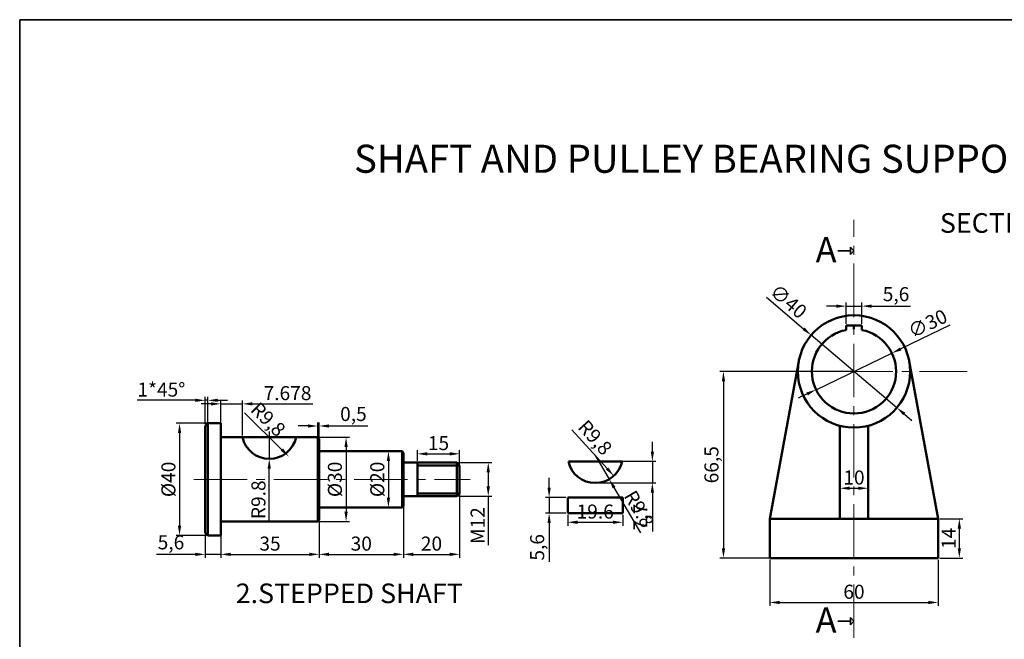
# Model space of a CAD drawing. Units: millimetres. Extents: x 54 to 669, y -108 to 325.
# Tile 2 of 3: x 54 to 404, y 104 to 325. Entities that reach past the tile are written whole.
import ezdxf

# ---------------------------------------------------------------- set-up
doc = ezdxf.new("R2010")
doc.units = ezdxf.units.MM
doc.linetypes.add('CENTER2', pattern=[28.575, 19.05, -3.175, 3.175, -3.175])
for name, color, linetype, lineweight in [('M-CNTR', 1, 'CENTER2', 18), ('M-DIMS', 2, 'Continuous', 25), ('M-OUTL', 7, 'Continuous', 50), ('M-SECT', 6, 'Continuous', 35), ('M-TEXT', 3, 'Continuous', 25), ('M-TTLB', 7, 'Continuous', 35)]:
    doc.layers.add(name, color=color, linetype=linetype, lineweight=lineweight)
doc.styles.get("Standard").update_dxf_attribs({"font": 'arial.ttf'})
doc.dimstyles.new('ISO-25', dxfattribs={"dimtxt": 5, "dimasz": 3.5, "dimexe": 1.25, "dimexo": 0.625, "dimtad": 1, "dimdec": 1, "dimtxsty": 'Standard', "dimcen": 2.5, "dimadec": 0, "dimazin": 0, "dimtfac": 1, "dimtdec": 1, "dimtmove": 0, "dimatfit": 3, "dimfxl": 1, "dimarcsym": 0})

# ---------------------------------------------------------------- blocks, each defined once
blk = doc.blocks.new('*U1')
at = {"layer": 'M-CNTR', "color": 0, "transparency": 16777216}
blk.add_line((-26.94, 0), (71.57, 0), dxfattribs=at)
blk = doc.blocks.new('*D2')
at = {"layer": 'Defpoints', "color": 0, "transparency": 16777216}
for p in [(119.67, 142.19), (125.27, 142.19), (125.27, 134.48)]:
    blk.add_point(p, dxfattribs=at)
at = {"layer": 'M-DIMS', "color": 0, "lineweight": -2, "transparency": 16777216}
for p, q in [((119.67, 141.57), (119.67, 133.23)), ((125.27, 141.57), (125.27, 133.23)), ((116.17, 134.48), (102.32, 134.48)), ((125.27, 134.48), (119.67, 134.48)), ((128.77, 134.48), (132.27, 134.48))]:
    blk.add_line(p, q, dxfattribs=at)
at = {"layer": 'M-DIMS', "color": 0, "transparency": 16777216}
for points in [[(116.17, 135.07), (116.17, 133.9), (119.67, 134.48)], [(128.77, 135.07), (128.77, 133.9), (125.27, 134.48)]]:
    blk.add_solid(points, dxfattribs=at)
at = {"layer": 'M-DIMS', "color": 0, "transparency": 16777216, "insert": (107.5, 138.11), "char_height": 5, "attachment_point": 5}
blk.add_mtext('5,6', dxfattribs=at)
blk = doc.blocks.new('*D3')
at = {"layer": 'Defpoints', "color": 0, "transparency": 16777216}
for p in [(125.27, 146.19), (160.27, 146.69), (160.27, 134.48)]:
    blk.add_point(p, dxfattribs=at)
at = {"layer": 'M-DIMS', "color": 0, "lineweight": -2, "transparency": 16777216}
for p, q in [((125.27, 145.57), (125.27, 133.23)), ((160.27, 146.07), (160.27, 133.23)), ((128.77, 134.48), (156.77, 134.48))]:
    blk.add_line(p, q, dxfattribs=at)
at = {"layer": 'M-DIMS', "color": 0, "transparency": 16777216}
for points in [[(128.77, 135.07), (128.77, 133.9), (125.27, 134.48)], [(156.77, 135.07), (156.77, 133.9), (160.27, 134.48)]]:
    blk.add_solid(points, dxfattribs=at)
at = {"layer": 'M-DIMS', "color": 0, "transparency": 16777216, "insert": (142.77, 137.66), "char_height": 5, "attachment_point": 5}
blk.add_mtext('35', dxfattribs=at)
blk = doc.blocks.new('*D4')
at = {"layer": 'Defpoints', "color": 0, "transparency": 16777216}
for p in [(190.27, 153.05), (160.27, 146.69), (190.27, 134.48)]:
    blk.add_point(p, dxfattribs=at)
at = {"layer": 'M-DIMS', "color": 0, "lineweight": -2, "transparency": 16777216}
for p, q in [((190.27, 152.43), (190.27, 133.23)), ((160.27, 146.07), (160.27, 133.23)), ((163.77, 134.48), (186.77, 134.48))]:
    blk.add_line(p, q, dxfattribs=at)
at = {"layer": 'M-DIMS', "color": 0, "transparency": 16777216}
for points in [[(163.77, 135.07), (163.77, 133.9), (160.27, 134.48)], [(186.77, 135.07), (186.77, 133.9), (190.27, 134.48)]]:
    blk.add_solid(points, dxfattribs=at)
at = {"layer": 'M-DIMS', "color": 0, "transparency": 16777216, "insert": (175.27, 137.66), "char_height": 5, "attachment_point": 5}
blk.add_mtext('30', dxfattribs=at)
blk = doc.blocks.new('*D5')
at = {"layer": 'Defpoints', "color": 0, "transparency": 16777216}
for p in [(210.27, 158.42), (190.27, 153.05), (210.27, 134.48)]:
    blk.add_point(p, dxfattribs=at)
at = {"layer": 'M-DIMS', "color": 0, "lineweight": -2, "transparency": 16777216}
for p, q in [((210.27, 157.8), (210.27, 133.23)), ((190.27, 152.43), (190.27, 133.23)), ((193.77, 134.48), (206.77, 134.48))]:
    blk.add_line(p, q, dxfattribs=at)
at = {"layer": 'M-DIMS', "color": 0, "transparency": 16777216}
for points in [[(193.77, 135.07), (193.77, 133.9), (190.27, 134.48)], [(206.77, 135.07), (206.77, 133.9), (210.27, 134.48)]]:
    blk.add_solid(points, dxfattribs=at)
at = {"layer": 'M-DIMS', "color": 0, "transparency": 16777216, "insert": (200.27, 137.66), "char_height": 5, "attachment_point": 5}
blk.add_mtext('20', dxfattribs=at)
blk = doc.blocks.new('*D6')
at = {"layer": 'Defpoints', "color": 0, "transparency": 16777216}
for p in [(122.97, 181.19), (110.55, 141.19), (120.67, 141.19)]:
    blk.add_point(p, dxfattribs=at)
at = {"layer": 'M-DIMS', "color": 0, "lineweight": -2, "transparency": 16777216}
for p, q in [((122.35, 181.19), (109.3, 181.19)), ((110.55, 177.69), (110.55, 144.69)), ((120.05, 141.19), (109.3, 141.19))]:
    blk.add_line(p, q, dxfattribs=at)
at = {"layer": 'M-DIMS', "color": 0, "transparency": 16777216}
for points in [[(109.97, 177.69), (111.13, 177.69), (110.55, 181.19)], [(109.97, 144.69), (111.13, 144.69), (110.55, 141.19)]]:
    blk.add_solid(points, dxfattribs=at)
at = {"layer": 'M-DIMS', "color": 0, "transparency": 16777216, "insert": (107.23, 161.19), "char_height": 5, "attachment_point": 5, "rotation": 90}
blk.add_mtext('%%C40', dxfattribs=at)
blk = doc.blocks.new('*D7')
at = {"layer": 'Defpoints', "color": 0, "transparency": 16777216}
for p in [(209.27, 167.19), (209.27, 155.19), (220.49, 155.19)]:
    blk.add_point(p, dxfattribs=at)
at = {"layer": 'M-DIMS', "color": 0, "lineweight": -2, "transparency": 16777216}
for p, q in [((209.9, 167.19), (221.74, 167.19)), ((220.49, 163.69), (220.49, 158.69)), ((209.9, 155.19), (221.74, 155.19)), ((220.49, 155.19), (220.49, 137.74))]:
    blk.add_line(p, q, dxfattribs=at)
at = {"layer": 'M-DIMS', "color": 0, "transparency": 16777216}
for points in [[(219.91, 163.69), (221.08, 163.69), (220.49, 167.19)], [(219.91, 158.69), (221.08, 158.69), (220.49, 155.19)]]:
    blk.add_solid(points, dxfattribs=at)
at = {"layer": 'M-DIMS', "color": 0, "transparency": 16777216, "insert": (217.36, 144.72), "char_height": 5, "attachment_point": 5, "rotation": 90}
blk.add_mtext('M12', dxfattribs=at)
blk = doc.blocks.new('*D8')
at = {"layer": 'Defpoints', "color": 0, "transparency": 16777216}
for p in [(142.52, 176.19), (149.5, 169.31)]:
    blk.add_point(p, dxfattribs=at)
at = {"layer": 'M-DIMS', "color": 0, "lineweight": -2, "transparency": 16777216}
blk.add_line((133.73, 184.86), (147.01, 171.77), dxfattribs=at)
at = {"layer": 'M-DIMS', "color": 0, "transparency": 16777216}
blk.add_solid([(147.42, 172.18), (146.6, 171.35), (149.5, 169.31)], dxfattribs=at)
at = {"layer": 'M-DIMS', "color": 0, "transparency": 16777216, "insert": (141.67, 182.13), "char_height": 5, "attachment_point": 5, "rotation": 315.3948}
blk.add_mtext('R9,8', dxfattribs=at)
blk = doc.blocks.new('*D9')
at = {"layer": 'Defpoints', "color": 0, "transparency": 16777216}
for p in [(160.27, 180.21), (159.77, 174.53), (160.27, 174.53)]:
    blk.add_point(p, dxfattribs=at)
at = {"layer": 'M-DIMS', "color": 0, "lineweight": -2, "transparency": 16777216}
for p, q in [((156.27, 180.21), (152.77, 180.21)), ((159.77, 175.16), (159.77, 181.46)), ((159.77, 180.21), (160.27, 180.21)), ((160.27, 175.16), (160.27, 181.46)), ((163.77, 180.21), (177.66, 180.21))]:
    blk.add_line(p, q, dxfattribs=at)
at = {"layer": 'M-DIMS', "color": 0, "transparency": 16777216}
for points in [[(156.27, 180.79), (156.27, 179.63), (159.77, 180.21)], [(163.77, 180.79), (163.77, 179.63), (160.27, 180.21)]]:
    blk.add_solid(points, dxfattribs=at)
at = {"layer": 'M-DIMS', "color": 0, "transparency": 16777216, "insert": (172.47, 183.84), "char_height": 5, "attachment_point": 5}
blk.add_mtext('0,5', dxfattribs=at)
blk = doc.blocks.new('*D10')
at = {"layer": 'Defpoints', "color": 0, "transparency": 16777216}
for p in [(120.67, 189.36), (119.67, 180.21), (120.67, 179.21)]:
    blk.add_point(p, dxfattribs=at)
at = {"layer": 'M-DIMS', "color": 0, "lineweight": -2, "transparency": 16777216}
for p, q in [((116.17, 189.36), (95.48, 189.36)), ((119.67, 180.83), (119.67, 190.61)), ((120.67, 189.36), (119.67, 189.36)), ((120.67, 179.83), (120.67, 190.61)), ((124.17, 189.36), (127.67, 189.36))]:
    blk.add_line(p, q, dxfattribs=at)
at = {"layer": 'M-DIMS', "color": 0, "transparency": 16777216}
for points in [[(116.17, 189.94), (116.17, 188.77), (119.67, 189.36)], [(124.17, 189.94), (124.17, 188.77), (120.67, 189.36)]]:
    blk.add_solid(points, dxfattribs=at)
at = {"layer": 'M-DIMS', "color": 0, "transparency": 16777216, "insert": (104.08, 192.53), "char_height": 5, "attachment_point": 5}
blk.add_mtext('1*45%%D', dxfattribs=at)
blk = doc.blocks.new('*D11')
at = {"layer": 'Defpoints', "color": 0, "transparency": 16777216}
for p in [(248.78, 154.75), (242.18, 149.15), (248.78, 149.15)]:
    blk.add_point(p, dxfattribs=at)
at = {"layer": 'M-DIMS', "color": 0, "lineweight": -2, "transparency": 16777216}
for p, q in [((242.18, 158.25), (242.18, 161.75)), ((248.16, 154.75), (240.93, 154.75)), ((242.18, 154.75), (242.18, 149.15)), ((248.16, 149.15), (240.93, 149.15)), ((242.18, 145.65), (242.18, 131.8))]:
    blk.add_line(p, q, dxfattribs=at)
at = {"layer": 'M-DIMS', "color": 0, "transparency": 16777216}
for points in [[(241.59, 158.25), (242.76, 158.25), (242.18, 154.75)], [(241.59, 145.65), (242.76, 145.65), (242.18, 149.15)]]:
    blk.add_solid(points, dxfattribs=at)
at = {"layer": 'M-DIMS', "color": 0, "transparency": 16777216, "insert": (238.55, 136.98), "char_height": 5, "attachment_point": 5, "rotation": 90}
blk.add_mtext('5,6', dxfattribs=at)
blk = doc.blocks.new('*D12')
at = {"layer": 'Defpoints', "color": 0, "transparency": 16777216}
for p in [(258.58, 167.62), (258.58, 159.92), (278.93, 159.92)]:
    blk.add_point(p, dxfattribs=at)
at = {"layer": 'M-DIMS', "color": 0, "lineweight": -2, "transparency": 16777216}
for p, q in [((278.93, 171.12), (278.93, 174.62)), ((259.21, 167.62), (280.18, 167.62)), ((278.93, 167.62), (278.93, 159.92)), ((259.21, 159.92), (280.18, 159.92)), ((278.93, 156.42), (278.93, 142.61))]:
    blk.add_line(p, q, dxfattribs=at)
at = {"layer": 'M-DIMS', "color": 0, "transparency": 16777216}
for points in [[(278.35, 171.12), (279.52, 171.12), (278.93, 167.62)], [(278.35, 156.42), (279.52, 156.42), (278.93, 159.92)]]:
    blk.add_solid(points, dxfattribs=at)
at = {"layer": 'M-DIMS', "color": 0, "transparency": 16777216, "insert": (275.32, 147.76), "char_height": 5, "attachment_point": 5, "rotation": 90}
blk.add_mtext('7,7', dxfattribs=at)
blk = doc.blocks.new('*D13')
at = {"layer": 'Defpoints', "color": 0, "transparency": 16777216}
for p in [(258.58, 169.72), (265.17, 162.46)]:
    blk.add_point(p, dxfattribs=at)
at = {"layer": 'M-DIMS', "color": 0, "lineweight": -2, "transparency": 16777216}
blk.add_line((250.28, 178.86), (262.82, 165.05), dxfattribs=at)
at = {"layer": 'M-DIMS', "color": 0, "transparency": 16777216}
blk.add_solid([(263.25, 165.45), (262.39, 164.66), (265.17, 162.46)], dxfattribs=at)
at = {"layer": 'M-DIMS', "color": 0, "transparency": 16777216, "insert": (258.06, 175.69), "char_height": 5, "attachment_point": 5, "rotation": 312.2342}
blk.add_mtext('R9,8', dxfattribs=at)
blk = doc.blocks.new('*U14')
at = {"layer": 'M-CNTR', "color": 0, "transparency": 16777216}
blk.add_line((0, -35.45), (0, 113.53), dxfattribs=at)
blk = doc.blocks.new('*U17')
at = {"layer": 'M-CNTR', "color": 0, "transparency": 16777216}
blk.add_line((-52.22, 0), (21.93, 0), dxfattribs=at)
blk = doc.blocks.new('*D18')
at = {"layer": 'Defpoints', "color": 0, "transparency": 16777216}
for p in [(345.73, 158.03), (355.73, 158.03), (355.73, 158.03)]:
    blk.add_point(p, dxfattribs=at)
at = {"layer": 'M-DIMS', "color": 0, "lineweight": -2, "transparency": 16777216}
for p, q in [((345.73, 158.65), (345.73, 159.28)), ((349.23, 158.03), (352.23, 158.03)), ((355.73, 158.65), (355.73, 159.28))]:
    blk.add_line(p, q, dxfattribs=at)
at = {"layer": 'M-DIMS', "color": 0, "transparency": 16777216}
for points in [[(349.23, 158.61), (349.23, 157.44), (345.73, 158.03)], [(352.23, 158.61), (352.23, 157.44), (355.73, 158.03)]]:
    blk.add_solid(points, dxfattribs=at)
at = {"layer": 'M-DIMS', "color": 0, "transparency": 16777216, "insert": (350.73, 161.21), "char_height": 5, "attachment_point": 5}
blk.add_mtext('10', dxfattribs=at)
blk = doc.blocks.new('*D19')
at = {"layer": 'Defpoints', "color": 0, "transparency": 16777216}
for p in [(350.73, 199.66), (304.25, 133.16), (350.73, 133.16)]:
    blk.add_point(p, dxfattribs=at)
at = {"layer": 'M-DIMS', "color": 0, "lineweight": -2, "transparency": 16777216}
for p, q in [((350.11, 199.66), (303, 199.66)), ((304.25, 196.16), (304.25, 136.66)), ((350.11, 133.16), (303, 133.16))]:
    blk.add_line(p, q, dxfattribs=at)
at = {"layer": 'M-DIMS', "color": 0, "transparency": 16777216}
for points in [[(303.67, 196.16), (304.84, 196.16), (304.25, 199.66)], [(303.67, 136.66), (304.84, 136.66), (304.25, 133.16)]]:
    blk.add_solid(points, dxfattribs=at)
at = {"layer": 'M-DIMS', "color": 0, "transparency": 16777216, "insert": (300.62, 166.41), "char_height": 5, "attachment_point": 5, "rotation": 90}
blk.add_mtext('66,5', dxfattribs=at)
blk = doc.blocks.new('*D20')
at = {"layer": 'Defpoints', "color": 0, "transparency": 16777216}
for p in [(320.73, 133.16), (380.73, 133.16), (380.73, 117.33)]:
    blk.add_point(p, dxfattribs=at)
at = {"layer": 'M-DIMS', "color": 0, "lineweight": -2, "transparency": 16777216}
for p, q in [((320.73, 132.53), (320.73, 116.08)), ((380.73, 132.53), (380.73, 116.08)), ((324.23, 117.33), (377.23, 117.33))]:
    blk.add_line(p, q, dxfattribs=at)
at = {"layer": 'M-DIMS', "color": 0, "transparency": 16777216}
for points in [[(324.23, 117.91), (324.23, 116.75), (320.73, 117.33)], [(377.23, 117.91), (377.23, 116.75), (380.73, 117.33)]]:
    blk.add_solid(points, dxfattribs=at)
at = {"layer": 'M-DIMS', "color": 0, "transparency": 16777216, "insert": (350.73, 120.51), "char_height": 5, "attachment_point": 5}
blk.add_mtext('60', dxfattribs=at)
blk = doc.blocks.new('*D21')
at = {"layer": 'Defpoints', "color": 0, "transparency": 16777216}
for p in [(380.73, 147.16), (380.73, 133.16), (388.25, 133.16)]:
    blk.add_point(p, dxfattribs=at)
at = {"layer": 'M-DIMS', "color": 0, "lineweight": -2, "transparency": 16777216}
for p, q in [((381.36, 147.16), (389.5, 147.16)), ((388.25, 143.66), (388.25, 136.66)), ((381.36, 133.16), (389.5, 133.16))]:
    blk.add_line(p, q, dxfattribs=at)
at = {"layer": 'M-DIMS', "color": 0, "transparency": 16777216}
for points in [[(387.67, 143.66), (388.83, 143.66), (388.25, 147.16)], [(387.67, 136.66), (388.83, 136.66), (388.25, 133.16)]]:
    blk.add_solid(points, dxfattribs=at)
at = {"layer": 'M-DIMS', "color": 0, "transparency": 16777216, "insert": (385.11, 140.16), "char_height": 5, "attachment_point": 5, "rotation": 90}
blk.add_mtext('14', dxfattribs=at)
blk = doc.blocks.new('*D22')
at = {"layer": 'Defpoints', "color": 0, "transparency": 16777216}
for p in [(335.47, 212.58), (366, 186.73)]:
    blk.add_point(p, dxfattribs=at)
at = {"layer": 'M-DIMS', "color": 0, "lineweight": -2, "transparency": 16777216}
for p, q in [((319.57, 226.05), (332.8, 214.84)), ((366, 186.73), (335.47, 212.58)), ((368.67, 184.47), (371.34, 182.21))]:
    blk.add_line(p, q, dxfattribs=at)
at = {"layer": 'M-DIMS', "color": 0, "transparency": 16777216}
for points in [[(333.18, 215.29), (332.42, 214.4), (335.47, 212.58)], [(369.05, 184.92), (368.29, 184.03), (366, 186.73)]]:
    blk.add_solid(points, dxfattribs=at)
at = {"layer": 'M-DIMS', "color": 0, "transparency": 16777216, "insert": (326.99, 224.11), "char_height": 5, "attachment_point": 5, "rotation": 319.7435}
blk.add_mtext('∅40', dxfattribs=at)
blk = doc.blocks.new('*D23')
at = {"layer": 'Defpoints', "color": 0, "transparency": 16777216}
for p in [(364.25, 206.16), (337.22, 193.15)]:
    blk.add_point(p, dxfattribs=at)
at = {"layer": 'M-DIMS', "color": 0, "lineweight": -2, "transparency": 16777216}
for p, q in [((384.91, 216.11), (367.4, 207.68)), ((337.22, 193.15), (364.25, 206.16)), ((334.07, 191.63), (330.91, 190.11))]:
    blk.add_line(p, q, dxfattribs=at)
at = {"layer": 'M-DIMS', "color": 0, "transparency": 16777216}
for points in [[(367.15, 208.21), (367.66, 207.16), (364.25, 206.16)], [(333.81, 192.16), (334.32, 191.11), (337.22, 193.15)]]:
    blk.add_solid(points, dxfattribs=at)
at = {"layer": 'M-DIMS', "color": 0, "transparency": 16777216, "insert": (377.24, 216.1), "char_height": 5, "attachment_point": 5, "rotation": 25.7055}
blk.add_mtext('∅30', dxfattribs=at)
blk = doc.blocks.new('*D24')
at = {"layer": 'Defpoints', "color": 0, "transparency": 16777216}
for p in [(353.53, 222.91), (347.93, 215.98), (353.53, 215.98)]:
    blk.add_point(p, dxfattribs=at)
at = {"layer": 'M-DIMS', "color": 0, "lineweight": -2, "transparency": 16777216}
for p, q in [((344.43, 222.91), (340.93, 222.91)), ((347.93, 216.6), (347.93, 224.16)), ((347.93, 222.91), (353.53, 222.91)), ((353.53, 216.6), (353.53, 224.16)), ((357.03, 222.91), (370.88, 222.91))]:
    blk.add_line(p, q, dxfattribs=at)
at = {"layer": 'M-DIMS', "color": 0, "transparency": 16777216}
for points in [[(344.43, 223.49), (344.43, 222.32), (347.93, 222.91)], [(357.03, 223.49), (357.03, 222.32), (353.53, 222.91)]]:
    blk.add_solid(points, dxfattribs=at)
at = {"layer": 'M-DIMS', "color": 0, "transparency": 16777216, "insert": (365.71, 226.54), "char_height": 5, "attachment_point": 5}
blk.add_mtext('5,6', dxfattribs=at)
blk = doc.blocks.new('*D37')
at = {"layer": 'Defpoints', "color": 0, "transparency": 16777216}
for p in [(159.77, 176.19), (159.77, 146.19), (169.85, 146.19)]:
    blk.add_point(p, dxfattribs=at)
at = {"layer": 'M-DIMS', "color": 0, "lineweight": -2, "transparency": 16777216}
for p, q in [((160.4, 176.19), (171.1, 176.19)), ((169.85, 172.69), (169.85, 149.69)), ((160.4, 146.19), (171.1, 146.19))]:
    blk.add_line(p, q, dxfattribs=at)
at = {"layer": 'M-DIMS', "color": 0, "transparency": 16777216}
for points in [[(169.27, 172.69), (170.44, 172.69), (169.85, 176.19)], [(169.27, 149.69), (170.44, 149.69), (169.85, 146.19)]]:
    blk.add_solid(points, dxfattribs=at)
at = {"layer": 'M-DIMS', "color": 0, "transparency": 16777216, "insert": (166.53, 161.19), "char_height": 5, "attachment_point": 5, "rotation": 90}
blk.add_mtext('%%C30', dxfattribs=at)
blk = doc.blocks.new('*D38')
at = {"layer": 'Defpoints', "color": 0, "transparency": 16777216}
for p in [(187.03, 171.19), (184.94, 151.19), (187.03, 151.19)]:
    blk.add_point(p, dxfattribs=at)
at = {"layer": 'M-DIMS', "color": 0, "lineweight": -2, "transparency": 16777216}
for p, q in [((186.41, 171.19), (183.69, 171.19)), ((184.94, 167.69), (184.94, 154.69)), ((186.41, 151.19), (183.69, 151.19))]:
    blk.add_line(p, q, dxfattribs=at)
at = {"layer": 'M-DIMS', "color": 0, "transparency": 16777216}
for points in [[(184.35, 167.69), (185.52, 167.69), (184.94, 171.19)], [(184.35, 154.69), (185.52, 154.69), (184.94, 151.19)]]:
    blk.add_solid(points, dxfattribs=at)
at = {"layer": 'M-DIMS', "color": 0, "transparency": 16777216, "insert": (181.62, 161.19), "char_height": 5, "attachment_point": 5, "rotation": 90}
blk.add_mtext('%%C20', dxfattribs=at)
blk = doc.blocks.new('*D39')
at = {"layer": 'Defpoints', "color": 0, "transparency": 16777216}
for p in [(210.27, 170.29), (195.27, 167.19), (210.27, 165.19)]:
    blk.add_point(p, dxfattribs=at)
at = {"layer": 'M-DIMS', "color": 0, "lineweight": -2, "transparency": 16777216}
for p, q in [((195.27, 167.82), (195.27, 171.54)), ((198.77, 170.29), (206.77, 170.29)), ((210.27, 165.82), (210.27, 171.54))]:
    blk.add_line(p, q, dxfattribs=at)
at = {"layer": 'M-DIMS', "color": 0, "transparency": 16777216}
for points in [[(198.77, 170.88), (198.77, 169.71), (195.27, 170.29)], [(206.77, 170.88), (206.77, 169.71), (210.27, 170.29)]]:
    blk.add_solid(points, dxfattribs=at)
at = {"layer": 'M-DIMS', "color": 0, "transparency": 16777216, "insert": (202.77, 173.47), "char_height": 5, "attachment_point": 5}
blk.add_mtext('15', dxfattribs=at)
blk = doc.blocks.new('SECTION-ARROW')
for p, q in [((349.46, 242.59), (344.98, 242.59)), ((350.73, 242.59), (349.46, 243.87)), ((349.46, 243.87), (349.46, 241.32)), ((350.73, 242.59), (349.46, 241.32))]:
    blk.add_line(p, q)
blk = doc.blocks.new('*D62')
at = {"layer": 'Defpoints', "color": 0, "transparency": 16777216}
for p in [(132.95, 188.09), (125.27, 176.19), (132.95, 176.19)]:
    blk.add_point(p, dxfattribs=at)
at = {"layer": 'M-DIMS', "color": 0, "lineweight": -2, "transparency": 16777216}
for p, q in [((121.77, 188.09), (118.27, 188.09)), ((125.27, 176.82), (125.27, 189.34)), ((125.27, 188.09), (132.95, 188.09)), ((132.95, 176.82), (132.95, 189.34)), ((136.45, 188.09), (158.04, 188.09))]:
    blk.add_line(p, q, dxfattribs=at)
at = {"layer": 'M-DIMS', "color": 0, "transparency": 16777216}
for points in [[(121.77, 188.68), (121.77, 187.51), (125.27, 188.09)], [(136.45, 188.68), (136.45, 187.51), (132.95, 188.09)]]:
    blk.add_solid(points, dxfattribs=at)
at = {"layer": 'M-DIMS', "color": 0, "transparency": 16777216, "insert": (149, 191.27), "char_height": 5, "attachment_point": 5}
blk.add_mtext('7.678', dxfattribs=at)
blk = doc.blocks.new('*D63')
at = {"layer": 'Defpoints', "color": 0, "transparency": 16777216}
for p in [(248.78, 149.15), (268.38, 149.15), (268.38, 145.9)]:
    blk.add_point(p, dxfattribs=at)
at = {"layer": 'M-DIMS', "color": 0, "lineweight": -2, "transparency": 16777216}
for p, q in [((248.78, 148.53), (248.78, 144.65)), ((268.38, 148.53), (268.38, 144.65)), ((252.28, 145.9), (264.88, 145.9))]:
    blk.add_line(p, q, dxfattribs=at)
at = {"layer": 'M-DIMS', "color": 0, "transparency": 16777216}
for points in [[(252.28, 146.49), (252.28, 145.32), (248.78, 145.9)], [(264.88, 146.49), (264.88, 145.32), (268.38, 145.9)]]:
    blk.add_solid(points, dxfattribs=at)
at = {"layer": 'M-DIMS', "color": 0, "transparency": 16777216, "insert": (258.58, 149.08), "char_height": 5, "attachment_point": 5}
blk.add_mtext('19.6', dxfattribs=at)
blk = doc.blocks.new('*D67')
at = {"layer": 'Defpoints', "color": 0, "transparency": 16777216}
for p in [(142.52, 178.29), (142.5, 168.49)]:
    blk.add_point(p, dxfattribs=at)
at = {"layer": 'M-DIMS', "color": 0, "lineweight": -2, "transparency": 16777216}
for p, q in [((142.52, 178.29), (142.5, 168.49)), ((142.45, 146.34), (142.49, 164.99))]:
    blk.add_line(p, q, dxfattribs=at)
at = {"layer": 'M-DIMS', "color": 0, "transparency": 16777216}
blk.add_solid([(141.91, 164.99), (143.08, 164.99), (142.5, 168.49)], dxfattribs=at)
at = {"layer": 'M-DIMS', "color": 0, "transparency": 16777216, "insert": (139.29, 153.93), "char_height": 5, "attachment_point": 5, "rotation": 89.8653}
blk.add_mtext('R9.8', dxfattribs=at)
blk = doc.blocks.new('*D68')
at = {"layer": 'Defpoints', "color": 0, "transparency": 16777216}
for p in [(258.58, 169.72), (263.55, 161.27)]:
    blk.add_point(p, dxfattribs=at)
at = {"layer": 'M-DIMS', "color": 0, "lineweight": -2, "transparency": 16777216}
for p, q in [((258.58, 169.72), (263.55, 161.27)), ((274.77, 142.17), (265.32, 158.25))]:
    blk.add_line(p, q, dxfattribs=at)
at = {"layer": 'M-DIMS', "color": 0, "transparency": 16777216}
blk.add_solid([(265.82, 158.55), (264.82, 157.95), (263.55, 161.27)], dxfattribs=at)
at = {"layer": 'M-DIMS', "color": 0, "transparency": 16777216, "insert": (273.67, 150.31), "char_height": 5, "attachment_point": 5, "rotation": 300.4294}
blk.add_mtext('R9.8', dxfattribs=at)

msp = doc.modelspace()

# ---------------------------------------------------------------- linework, layer by layer
at = {"layer": 'M-OUTL'}
for p, q in [((347.9346, 215.9769), (347.9346, 214.3932)), ((353.5346, 215.9769), (347.9346, 215.9769)), ((350.7346, 215.9769), (350.7346, 214.6569)), ((353.5346, 215.9769), (353.5346, 214.3932)), ((331.0651, 203.2776), (320.7346, 147.1569)), ((370.4041, 203.2776), (380.7346, 147.1569)), ((120.673, 181.1917), (119.673, 180.1917)), ((119.673, 180.1917), (119.673, 142.1917)), ((125.273, 181.1917), (120.673, 181.1917)), ((120.673, 181.1917), (120.673, 141.1917)), ((125.273, 141.1917), (125.273, 181.1917)), ((345.7346, 147.1569), (345.7346, 180.292)), ((355.7346, 147.1569), (355.7346, 180.292)), ((125.273, 176.1917), (159.773, 176.1917)), ((159.773, 176.1917), (159.773, 146.1917)), ((160.273, 175.6917), (159.773, 176.1917)), ((160.273, 175.6917), (160.273, 146.6917)), ((160.273, 171.1917), (189.773, 171.1917)), ((189.773, 171.1917), (189.773, 151.1917)), ((190.273, 170.6917), (189.773, 171.1917)), ((190.273, 170.6917), (190.273, 151.6917)), ((190.273, 167.1917), (209.273, 167.1917)), ((195.273, 167.1917), (195.273, 155.1917)), ((195.273, 166.1917), (210.273, 166.1917)), ((209.273, 167.1917), (209.273, 155.1917)), ((209.273, 167.1917), (210.273, 166.1917)), ((210.273, 166.1917), (210.273, 156.1917)), ((249.0117, 167.618), (268.1564, 167.618)), ((209.273, 155.1917), (190.273, 155.1917)), ((210.273, 156.1917), (195.273, 156.1917)), ((210.273, 156.1917), (209.273, 155.1917)), ((248.784, 154.7525), (268.384, 154.7525)), ((248.784, 149.1525), (248.784, 154.7525)), ((268.384, 154.7525), (268.384, 149.1525)), ((189.773, 151.1917), (160.273, 151.1917)), ((190.273, 151.6917), (189.773, 151.1917)), ((268.384, 149.1525), (248.784, 149.1525)), ((159.773, 146.1917), (125.273, 146.1917)), ((160.273, 146.6917), (159.773, 146.1917)), ((380.7346, 147.1569), (320.7346, 147.1569)), ((320.7346, 147.1569), (320.7346, 133.1569)), ((380.7346, 133.1569), (380.7346, 147.1569)), ((119.673, 142.1917), (120.673, 141.1917)), ((120.673, 141.1917), (125.273, 141.1917)), ((320.7346, 133.1569), (380.7346, 133.1569))]:
    msp.add_line(p, q, dxfattribs=at)
msp.add_lwpolyline([(152.0954, 176.1917), (132.9507, 176.1917, 0.80439967)], format="xyb", close=True, dxfattribs=at)
msp.add_circle((350.7346, 199.6569), 20, dxfattribs=at)
for centre, radius, start, end in [((350.7346, 199.6569), 15, 100.758318, 79.241682), ((258.584, 169.718), 9.8, 192.373625, 347.626375)]:
    msp.add_arc(centre, radius, start, end, dxfattribs=at)
at = {"layer": 'M-TTLB'}
msp.add_lwpolyline([(53.6241, 324.969), (668.8363, 324.969), (668.8363, -108.3789), (53.6241, -108.3789)], close=True, dxfattribs=at)

# ---------------------------------------------------------------- block references
at = {"layer": 'M-CNTR'}
for name, p in [('*U14', (350.7346, 140.1569)), ('*U17', (369.1611, 199.6569)), ('*U1', (142.523, 161.1917))]:
    msp.add_blockref(name, p, dxfattribs=at)
at = {"layer": 'M-SECT'}
for p in [(0, 0), (0, -131.9304)]:
    msp.add_blockref('SECTION-ARROW', p, dxfattribs=at)

# ---------------------------------------------------------------- texts
at = {"layer": 'M-TEXT', "attachment_point": 1}
for s, width, insert, char_height in [('\\pxqc;SHAFT AND PULLEY BEARING SUPPORT ASSEMBLY', 425.505879, (120.0251, 280.4197), 10), ('SECTION A-A', 90.278815, (381.3251, 256.0386), 7), ('A', 11.75906, (337.0733, 247.5079), 9), ('2.STEPPED SHAFT', 90.278815, (130.5604, 124.0915), 7), ('A', 11.75906, (337.0733, 115.5775), 9)]:
    msp.add_mtext_dynamic_manual_height_columns(s, width=width, gutter_width=12.5, heights=[0], dxfattribs=dict(at, insert=insert, char_height=char_height))

# ---------------------------------------------------------------- dimensions: what is measured, and where the dimension line sits
at = {"layer": 'M-DIMS'}
dim = msp.add_diameter_dim_2p(p1=(365.9978, 186.7327), p2=(335.4714, 212.5811), dimstyle='ISO-25', override={"dimclrd": 0, "dimclre": 0, "dimclrt": 0}, dxfattribs=at)
dim.commit()
dim.dimension.update_dxf_attribs({"geometry": '*D22', "text_midpoint": (326.994, 224.1068)})
for base, p1, p2, override, picture, middle in [((353.5346, 222.9073), (347.9346, 215.9769), (353.5346, 215.9769), {"dimclrd": 0, "dimclre": 0, "dimclrt": 0}, '*D24', (365.7094, 226.5371)), ((132.9507, 188.0917), (125.273, 176.1917), (132.9507, 176.1917), {"dimdec": 3, "dimlfac": 1, "dimrnd": 0, "dimzin": 0, "dimdsep": 46, "dimlunit": 2}, '*D62', (148.9965, 191.2696)), ((160.273, 180.209), (159.773, 174.5346), (160.273, 174.5346), {"dimclrd": 0, "dimclre": 0, "dimclrt": 0}, '*D9', (172.4683, 183.8387)), ((210.273, 170.2948), (195.273, 167.1917), (210.273, 165.1917), {"dimclrd": 0, "dimclre": 0, "dimclrt": 0}, '*D39', (202.773, 173.4727)), ((355.7346, 158.0274), (345.7346, 158.0274), (355.7346, 158.0274), {"dimclrd": 0, "dimclre": 0, "dimclrt": 0}, '*D18', (350.7346, 161.2053)), ((268.384, 145.9025), (248.784, 149.1525), (268.384, 149.1525), {"dimdec": 1, "dimlfac": 1, "dimrnd": 0, "dimzin": 0, "dimdsep": 46, "dimlunit": 2}, '*D63', (258.584, 149.0803)), ((160.273, 134.4848), (125.273, 146.1917), (160.273, 146.6917), {"dimclrd": 0, "dimclre": 0, "dimclrt": 0, "dimtmove": 0}, '*D3', (142.773, 137.6643)), ((380.7346, 117.3303), (320.7346, 133.1569), (380.7346, 133.1569), {"dimclrd": 0, "dimclre": 0, "dimclrt": 0}, '*D20', (350.7346, 120.5081))]:
    dim = msp.add_linear_dim(base=base, p1=p1, p2=p2, dimstyle='ISO-25', override=override, dxfattribs=at)
    dim.commit()
    dim.dimension.update_dxf_attribs({"geometry": picture, "text_midpoint": middle})
dim = msp.add_diameter_dim_2p(p1=(337.2191, 193.1507), p2=(364.2501, 206.1631), dimstyle='ISO-25', override={"dimclrd": 0, "dimclre": 0, "dimclrt": 0}, dxfattribs=at)
dim.commit()
dim.dimension.update_dxf_attribs({"geometry": '*D23', "text_midpoint": (378.6748, 213.1069), "dimtype": 163})
for base, p1, p2, picture, middle in [((304.2528, 133.1569), (350.7346, 199.6569), (350.7346, 133.1569), '*D19', (300.623, 166.4069)), ((278.9349, 159.918), (258.584, 167.618), (258.584, 159.918), '*D12', (275.3154, 147.762)), ((242.1753, 149.1525), (248.784, 154.7525), (248.784, 149.1525), '*D11', (238.5456, 136.9777)), ((388.2496, 133.1569), (380.7346, 147.1569), (380.7346, 133.1569), '*D21', (385.1144, 140.1569))]:
    dim = msp.add_linear_dim(base=base, p1=p1, p2=p2, angle=90, dimstyle='ISO-25', override={"dimclrd": 0, "dimclre": 0, "dimclrt": 0}, dxfattribs=at)
    dim.commit()
    dim.dimension.update_dxf_attribs({"geometry": picture, "text_midpoint": middle})
dim = msp.add_linear_dim(base=(120.673, 189.3566), p1=(119.673, 180.209), p2=(120.673, 179.209), text='<>*45%%D', dimstyle='ISO-25', override={"dimclrd": 0, "dimclre": 0, "dimclrt": 0}, dxfattribs=at)
dim.commit()
dim.dimension.update_dxf_attribs({"geometry": '*D10', "text_midpoint": (104.0774, 189.3566), "dimtype": 160})
for center, mpoint, picture, middle in [((142.523, 176.1917), (149.5003, 169.31), '*D8', (139.124, 179.5442)), ((258.584, 169.718), (265.1712, 162.4621), '*D13', (255.375, 173.2529))]:
    dim = msp.add_radius_dim(center=center, mpoint=mpoint, dimstyle='ISO-25', override={"dimclrd": 0, "dimclre": 0, "dimclrt": 0}, dxfattribs=at)
    dim.commit()
    dim.dimension.update_dxf_attribs({"geometry": picture, "text_midpoint": middle, "dimtype": 164})
for base, p1, p2, text, picture, middle in [((110.5507, 141.1917), (122.973, 181.1917), (120.673, 141.1917), '%%C<>', '*D6', (107.233, 161.1917)), ((169.8519, 146.1917), (159.773, 176.1917), (159.773, 146.1917), '%%C<>', '*D37', (166.5342, 161.1917)), ((184.9354, 151.1917), (187.0346, 171.1917), (187.0346, 151.1917), '%%C<>', '*D38', (181.6177, 161.1917)), ((220.493, 155.1917), (209.273, 167.1917), (209.273, 155.1917), 'M<>', '*D7', (217.3578, 144.7161))]:
    dim = msp.add_linear_dim(base=base, p1=p1, p2=p2, angle=90, text=text, dimstyle='ISO-25', override={"dimclrd": 0, "dimclre": 0, "dimclrt": 0}, dxfattribs=at)
    dim.commit()
    dim.dimension.update_dxf_attribs({"geometry": picture, "text_midpoint": middle})
for center, mpoint, picture, middle in [((142.523, 178.2917), (142.5, 168.4917), '*D67', (139.2879, 153.9251)), ((258.584, 169.718), (263.5475, 161.268), '*D68', (273.6691, 150.3108))]:
    dim = msp.add_radius_dim(center=center, mpoint=mpoint, dimstyle='ISO-25', override={"dimdec": 1, "dimlfac": 1, "dimrnd": 0, "dimzin": 0, "dimdsep": 46, "dimlunit": 2}, dxfattribs=at)
    dim.commit()
    dim.dimension.update_dxf_attribs({"geometry": picture, "text_midpoint": middle})
for base, p1, p2, override, picture, middle in [((210.273, 134.4848), (190.273, 153.0546), (210.273, 158.4225), {"dimclrd": 0, "dimclre": 0, "dimclrt": 0, "dimtmove": 0}, '*D5', (200.273, 134.4848)), ((190.273, 134.4848), (160.273, 146.6917), (190.273, 153.0546), {"dimclrd": 0, "dimclre": 0, "dimclrt": 0, "dimtmove": 0}, '*D4', (175.273, 134.4848)), ((125.273, 134.4848), (119.673, 142.1917), (125.273, 142.1917), {"dimclrd": 0, "dimclre": 0, "dimclrt": 0}, '*D2', (107.4982, 134.4848))]:
    dim = msp.add_linear_dim(base=base, p1=p1, p2=p2, dimstyle='ISO-25', override=override, dxfattribs=at)
    dim.commit()
    dim.dimension.update_dxf_attribs({"geometry": picture, "text_midpoint": middle, "dimtype": 160})

doc.saveas('drawing.dxf')
